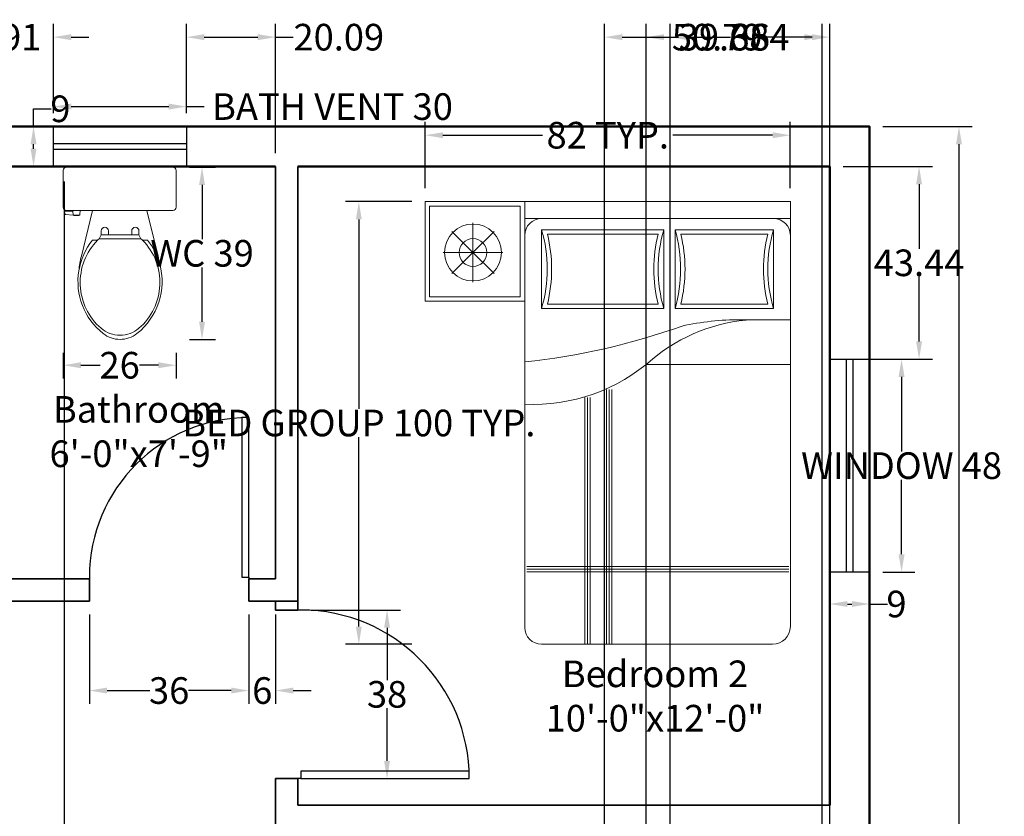
# Model space of a CAD drawing. Units: inches. Extents: x 89 to 490, y -59 to 378.
# Tile 20 of 20: x 268 to 490, y 198 to 378. Entities that reach past the tile are written whole.
import ezdxf

# ---------------------------------------------------------------- set-up
doc = ezdxf.new("R2010")
doc.units = ezdxf.units.IN
doc.header["$MEASUREMENT"] = 0
for name, color, linetype, lineweight in [('A-ANNO-DIMS', 2, 'Continuous', 18), ('A-AREA-IDEN', 7, 'Continuous', 18), ('Beds', 64, 'Continuous', 18), ('Commode', 232, 'Continuous', 18), ('Doors', 34, 'Continuous', 25), ('Inner Walls', 31, 'Continuous', 35), ('Outer Walls', 12, 'Continuous', 50), ('Ventilators', 130, 'Continuous', 25), ('Windows', 171, 'Continuous', 25)]:
    doc.layers.add(name, color=color, linetype=linetype, lineweight=lineweight)
doc.styles.get("Standard").update_dxf_attribs({"font": 'arial.ttf'})
doc.dimstyles.get("Standard").update_dxf_attribs({"dimtxt": 6, "dimasz": 4, "dimexe": 3, "dimexo": 3, "dimgap": 0.09, "dimtad": 0, "dimtih": 1, "dimtoh": 1, "dimdec": 1, "dimzin": 0, "dimdsep": 46, "dimlunit": 3, "dimtxsty": 'Standard', "dimcen": 0.09, "dimadec": 0, "dimazin": 0, "dimtfac": 1, "dimtdec": 1, "dimtofl": 0, "dimtmove": 0, "dimatfit": 3, "dimfxl": 1, "dimtolj": 1, "dimtzin": 0, "dimarcsym": 0})

# ---------------------------------------------------------------- blocks, each defined once
blk = doc.blocks.new('Ventilator')
for p, q in [((814.98, 322.93), (844.98, 322.93)), ((814.98, 313.93), (814.98, 322.93)), ((844.98, 322.93), (844.98, 313.93)), ((814.98, 319.13), (844.98, 319.13)), ((844.98, 317.73), (814.98, 317.73)), ((844.98, 313.93), (814.98, 313.93))]:
    blk.add_line(p, q)
blk = doc.blocks.new('Window 1.1')
for p, q in [((642.96, 338.61), (642.96, 386.61)), ((644.36, 386.61), (644.36, 338.61))]:
    blk.add_line(p, q)
blk.add_lwpolyline([(648.16, 338.61), (639.16, 338.61), (639.16, 386.61), (648.16, 386.61)], close=True)
blk = doc.blocks.new('*U8')
for p, q in [((0, 0), (0, 6)), ((40, 0), (40, 6))]:
    blk.add_line(p, q)
blk.add_lwpolyline([(0, 0), (0, -40), (1.75, -40), (1.75, 0)], close=True)
blk.add_arc((0, 0), 40, 270, 0)
blk = doc.blocks.new('*U7')
for p, q in [((0, 0), (0, -6)), ((-40, 0), (-40, -6))]:
    blk.add_line(p, q)
blk.add_lwpolyline([(0, 0), (0, 40), (-1.75, 40), (-1.75, 0)], close=True)
blk.add_arc((0, 0), 40, 90, 180)
blk = doc.blocks.new('A$C216962CD')
at = {"linetype": 'ByBlock'}
for p, q in [((0, 1.5502), (0, 2.0002)), ((0, 2.0002), (0.45, 2.0002)), ((0.45, 1.924), (0.45, 2.0002)), ((0.45, 2.0002), (0.45, 1.5502)), ((0.45, 2.0002), (1.6506, 2.0002)), ((1.6506, 2.0002), (1.6506, 1.5502)), ((0.45, 1.924), (1.6506, 1.924)), ((0.5262, 1.8732), (0.5262, 1.5176)), ((1.0785, 1.8732), (0.5262, 1.8732)), ((1.0785, 1.5176), (1.0785, 1.8732)), ((1.1293, 1.8732), (1.1293, 1.5176)), ((1.5744, 1.8732), (1.1293, 1.8732)), ((1.5744, 1.5176), (1.5744, 1.8732)), ((0.45, 0.0762), (0.45, 1.8478)), ((1.6506, 1.8478), (1.6506, 0.08)), ((0.45, 1.5502), (0, 1.5502)), ((0.5262, 1.5176), (1.0785, 1.5176)), ((1.1293, 1.5176), (1.5744, 1.5176)), ((1.4247, 1.4668), (1.6506, 1.4668)), ((1.0023, 1.2636), (1.6506, 1.2636)), ((1.5706, 0), (0.5262, 0))]:
    blk.add_line(p, q, dxfattribs=at)
for p, q in [((0.02, 1.5702), (0.02, 1.9802)), ((0.02, 1.9802), (0.43, 1.9802)), ((0.43, 1.9802), (0.43, 1.5702)), ((0.216, 1.7702), (0.216, 1.9046)), ((0.216, 1.7702), (0.121, 1.8652)), ((0.216, 1.7702), (0.3111, 1.8652)), ((1.0524, 1.8532), (0.5523, 1.8532)), ((1.5483, 1.8532), (1.1554, 1.8532)), ((0.216, 1.7702), (0.0817, 1.7702)), ((0.216, 1.7702), (0.121, 1.6752)), ((0.216, 1.7702), (0.216, 1.6358)), ((0.216, 1.7702), (0.3504, 1.7702)), ((0.216, 1.7702), (0.3111, 1.6752)), ((0.43, 1.5702), (0.02, 1.5702)), ((0.5523, 1.5376), (1.0524, 1.5376)), ((1.1554, 1.5376), (1.5483, 1.5376)), ((0.722, 1.1146), (0.722, 0)), ((0.734, 1.1146), (0.734, 0)), ((0.746, 1.1146), (0.746, 0)), ((0.8202, 1.1507), (0.8202, 0)), ((0.8322, 1.1507), (0.8322, 0)), ((0.8442, 1.1507), (0.8442, 0)), ((0.4599, 0.3521), (1.6437, 0.3521)), ((0.4599, 0.3401), (1.6437, 0.3401)), ((0.4599, 0.3281), (1.6437, 0.3281))]:
    blk.add_line(p, q)
for radius in [0.1285, 0.0628]:
    blk.add_circle((0.216, 1.7702), radius)
for centre, radius, start, end in [((0.5262, 1.8478), 0.0762, 90, 180), ((1.5744, 1.8478), 0.0762, 0, 90), ((-0.0834, 1.6954), 0.635, 343.7398, 16.2602), ((1.6881, 1.6954), 0.635, 163.7398, 196.2602), ((0.5197, 1.6954), 0.635, 343.7398, 16.2602), ((2.184, 1.6954), 0.635, 163.7398, 196.2602), ((0.1309, 4.3115), 3.0525, 275.9977, 289.7225), ((1.5209, 0.6982), 0.7696, 92.9261, 129.8555), ((1.4243, 0.2475), 1.2193, 89.9814, 102.4667), ((0.4856, 1.9017), 0.8181, 267.5082, 311.5038), ((0.5262, 0.0762), 0.0762, 180, 270), ((1.5706, 0.08), 0.08, 270, 0)]:
    blk.add_arc(centre, radius, start, end, dxfattribs=at)
for centre, start, end in [((-0.0834, 1.6954), 346.0594, 13.9406), ((1.6881, 1.6954), 166.0594, 193.9406), ((0.5197, 1.6954), 346.0594, 13.9406), ((2.184, 1.6954), 166.0594, 193.9406)]:
    blk.add_arc(centre, 0.655, start, end)
blk = doc.blocks.new('B1')
at = {"color": 0}
for p, q in [((0, 0), (-240, 0)), ((240, 0), (0, 0)), ((-255, -15), (-255, -180)), ((255, -180), (255, -15)), ((-212, -198.4), (-250.1, -198.4)), ((-250.1, -198.4), (-245.5, -212.1)), ((-243.7, -213.5), (-210.1, -215.4)), ((-240, -195), (-212.3, -195)), ((-212.3, -195), (-177.6, -195)), ((-212.3, -195), (-212, -198.4)), ((-212, -198.4), (-210.1, -215.4)), ((-206.1, -215.4), (-210.1, -215.4)), ((-206.1, -215.4), (-205.1, -217.4)), ((-184.1, -215.4), (-206.1, -215.4)), ((-185.1, -217.4), (-205.1, -217.4)), ((-184.1, -215.4), (-185.1, -217.4)), ((-181.8, -215.4), (-184.1, -215.4)), ((-177.6, -195), (-179.8, -213.7)), ((-177.6, -195), (-122, -195)), ((-122, -195), (-172.9, -400.4)), ((0, -195), (-122, -195)), ((122, -195), (0, -195)), ((172.9, -400.4), (122, -195)), ((122, -195), (240, -195)), ((-92.8, -322.2), (-83.7, -305.5)), ((-83.7, -305.5), (-83.7, -287.2)), ((-50.9, -305.5), (-83.7, -305.5)), ((-50.9, -287.2), (-50.9, -305.5)), ((1.6, -305.5), (-50.9, -305.5)), ((1.6, -305.5), (54.2, -305.5)), ((54.2, -287.2), (54.2, -305.5)), ((54.2, -305.5), (86.9, -305.5)), ((86.9, -305.5), (86.9, -287.2)), ((96.1, -322.2), (86.9, -305.5)), ((-99.8, -329.1), (-122.6, -329.1)), ((1.6, -322.2), (-92.8, -322.2)), ((1.6, -322.2), (96.1, -322.2)), ((103.1, -329.1), (125.8, -329.1))]:
    blk.add_line(p, q, dxfattribs=at)
for centre, radius, start, end in [((-240, -15), 15, 90, 180), ((240, -15), 15, 360, 90), ((-240, -180), 15, 180, 270), ((-243.6, -211.5), 2, 198.4349, 266.7295), ((-181.8, -213.4), 2, 270, 353.0073), ((240, -180), 15, 270, 0), ((-67.3, -287.2), 16.4, 0, 180), ((70.6, -287.2), 16.4, 0, 180), ((110.1, -515.7), 298.3, 141.274, 170.4901), ((93.8, -520.1), 272, 135.3828, 229.2681), ((93.8, -520.1), 272, 133.3236, 135.3828), ((-90.5, -520.1), 272, 310.7319, 44.6172), ((-90.5, -520.1), 272, 44.6172, 46.6764), ((-106.9, -515.7), 298.3, 15.5851, 38.726), ((175, -492.8), 360, 165.1314, 175.7954), ((-106.9, -515.7), 298.3, 308.2583, 15.5851), ((-175, -492.8), 360, 9.1506, 14.8686), ((110.1, -515.7), 298.3, 170.4901, 231.7417), ((0.1, -628.9), 128.5, 229.2681, 270.6684), ((1.7, -653.2), 123.1, 231.7417, 269.9885), ((3.1, -628.9), 128.5, 269.3316, 310.7319), ((1.6, -653.2), 123.1, 270.0115, 308.2583)]:
    blk.add_arc(centre, radius, start, end, dxfattribs=at)
blk = doc.blocks.new('*D24')
at = {"layer": 'A-ANNO-DIMS', "color": 0, "lineweight": -2, "transparency": 16777216}
for p, q in [((306.03, 344.57), (311.86, 344.57)), ((308.86, 340.57), (308.86, 328.35)), ((308.86, 309.75), (308.86, 321.96)), ((306.03, 305.75), (311.86, 305.75))]:
    blk.add_line(p, q, dxfattribs=at)
at = {"layer": 'A-ANNO-DIMS', "color": 0, "transparency": 16777216}
for points in [[(308.19, 340.57), (309.52, 340.57), (308.86, 344.57)], [(308.19, 309.75), (309.52, 309.75), (308.86, 305.75)]]:
    blk.add_solid(points, dxfattribs=at)
at = {"layer": 'Defpoints', "color": 0, "transparency": 16777216}
for p in [(303.03, 344.57), (308.86, 344.57), (303.03, 305.75)]:
    blk.add_point(p, dxfattribs=at)
at = {"layer": 'A-ANNO-DIMS', "color": 0, "transparency": 16777216, "insert": (308.86, 325.16), "char_height": 6, "attachment_point": 5}
blk.add_mtext('\\A1;WC 39', dxfattribs=at)
blk = doc.blocks.new('*D25')
at = {"layer": 'A-ANNO-DIMS', "color": 0, "lineweight": -2, "transparency": 16777216}
for p, q in [((277.53, 302.75), (277.53, 296.93)), ((303.03, 302.75), (303.03, 296.93)), ((281.53, 299.93), (285.85, 299.93)), ((299.03, 299.93), (294.72, 299.93))]:
    blk.add_line(p, q, dxfattribs=at)
at = {"layer": 'A-ANNO-DIMS', "color": 0, "transparency": 16777216}
for points in [[(281.53, 300.6), (281.53, 299.26), (277.53, 299.93)], [(299.03, 300.6), (299.03, 299.26), (303.03, 299.93)]]:
    blk.add_solid(points, dxfattribs=at)
at = {"layer": 'Defpoints', "color": 0, "transparency": 16777216}
for p in [(277.53, 305.75), (303.03, 305.75), (303.03, 299.93)]:
    blk.add_point(p, dxfattribs=at)
at = {"layer": 'A-ANNO-DIMS', "color": 0, "transparency": 16777216, "insert": (290.28, 299.93), "char_height": 6, "attachment_point": 5}
blk.add_mtext('\\A1;26', dxfattribs=at)
blk = doc.blocks.new('*D26')
at = {"layer": 'A-ANNO-DIMS', "color": 0, "lineweight": -2, "transparency": 16777216}
for p, q in [((275.35, 356.74), (275.35, 361.24)), ((305.35, 356.74), (305.35, 361.24)), ((279.35, 358.24), (301.35, 358.24)), ((305.35, 358.24), (309.35, 358.24))]:
    blk.add_line(p, q, dxfattribs=at)
at = {"layer": 'A-ANNO-DIMS', "color": 0, "transparency": 16777216}
for points in [[(279.35, 358.91), (279.35, 357.57), (275.35, 358.24)], [(301.35, 358.91), (301.35, 357.57), (305.35, 358.24)]]:
    blk.add_solid(points, dxfattribs=at)
at = {"layer": 'Defpoints', "color": 0, "transparency": 16777216}
for p in [(305.35, 358.24), (275.35, 353.74), (305.35, 353.74)]:
    blk.add_point(p, dxfattribs=at)
at = {"layer": 'A-ANNO-DIMS', "color": 0, "transparency": 16777216, "insert": (338.28, 358.24), "char_height": 6, "attachment_point": 5}
blk.add_mtext('\\A1;BATH VENT 30', dxfattribs=at)
blk = doc.blocks.new('*D27')
at = {"layer": 'A-ANNO-DIMS', "color": 0, "lineweight": -2, "transparency": 16777216}
for p, q in [((270.85, 353.74), (270.85, 357.74)), ((270.85, 357.74), (274.85, 357.74)), ((272.35, 353.74), (267.85, 353.74)), ((270.85, 348.74), (270.85, 349.74)), ((272.35, 344.74), (267.85, 344.74))]:
    blk.add_line(p, q, dxfattribs=at)
at = {"layer": 'A-ANNO-DIMS', "color": 0, "transparency": 16777216}
for points in [[(270.18, 349.74), (271.52, 349.74), (270.85, 353.74)], [(270.18, 348.74), (271.52, 348.74), (270.85, 344.74)]]:
    blk.add_solid(points, dxfattribs=at)
at = {"layer": 'Defpoints', "color": 0, "transparency": 16777216}
for p in [(270.85, 353.74), (275.35, 353.74), (275.35, 344.74)]:
    blk.add_point(p, dxfattribs=at)
at = {"layer": 'A-ANNO-DIMS', "color": 0, "transparency": 16777216, "insert": (276.91, 357.74), "char_height": 6, "attachment_point": 5}
blk.add_mtext('\\A1;9', dxfattribs=at)
blk = doc.blocks.new('*D30')
at = {"layer": 'A-ANNO-DIMS', "color": 0, "lineweight": -2, "transparency": 16777216}
for p, q in [((356.2, 336.82), (341.22, 336.82)), ((344.22, 332.82), (344.22, 290.11)), ((344.22, 241.01), (344.22, 283.72)), ((356.2, 237.01), (341.22, 237.01))]:
    blk.add_line(p, q, dxfattribs=at)
at = {"layer": 'A-ANNO-DIMS', "color": 0, "transparency": 16777216}
for points in [[(343.56, 332.82), (344.89, 332.82), (344.22, 336.82)], [(343.56, 241.01), (344.89, 241.01), (344.22, 237.01)]]:
    blk.add_solid(points, dxfattribs=at)
at = {"layer": 'Defpoints', "color": 0, "transparency": 16777216}
for p in [(344.22, 336.82), (359.2, 336.82), (359.2, 237.01)]:
    blk.add_point(p, dxfattribs=at)
at = {"layer": 'A-ANNO-DIMS', "color": 0, "transparency": 16777216, "insert": (344.22, 286.91), "char_height": 6, "attachment_point": 5}
blk.add_mtext('\\A1;BED GROUP 100 TYP.', dxfattribs=at)
blk = doc.blocks.new('*D31')
at = {"layer": 'A-ANNO-DIMS', "color": 0, "lineweight": -2, "transparency": 16777216}
for p, q in [((359.2, 339.82), (359.2, 354.79)), ((441.55, 339.82), (441.55, 354.79)), ((363.2, 351.79), (385.68, 351.79)), ((437.55, 351.79), (415.07, 351.79))]:
    blk.add_line(p, q, dxfattribs=at)
at = {"layer": 'A-ANNO-DIMS', "color": 0, "transparency": 16777216}
for points in [[(363.2, 352.45), (363.2, 351.12), (359.2, 351.79)], [(437.55, 352.45), (437.55, 351.12), (441.55, 351.79)]]:
    blk.add_solid(points, dxfattribs=at)
at = {"layer": 'Defpoints', "color": 0, "transparency": 16777216}
for p in [(441.55, 351.79), (359.2, 336.82), (441.55, 336.82)]:
    blk.add_point(p, dxfattribs=at)
at = {"layer": 'A-ANNO-DIMS', "color": 0, "transparency": 16777216, "insert": (400.37, 351.79), "char_height": 6, "attachment_point": 5}
blk.add_mtext('\\A1;82 TYP.', dxfattribs=at)
blk = doc.blocks.new('*D34')
at = {"layer": 'A-ANNO-DIMS', "color": 0, "lineweight": -2, "transparency": 16777216}
for p, q in [((462.44, 301.3), (469.64, 301.3)), ((466.64, 297.3), (466.64, 280.49)), ((466.64, 257.3), (466.64, 274.11)), ((462.44, 253.3), (469.64, 253.3))]:
    blk.add_line(p, q, dxfattribs=at)
at = {"layer": 'A-ANNO-DIMS', "color": 0, "transparency": 16777216}
for points in [[(465.97, 297.3), (467.31, 297.3), (466.64, 301.3)], [(465.97, 257.3), (467.31, 257.3), (466.64, 253.3)]]:
    blk.add_solid(points, dxfattribs=at)
at = {"layer": 'Defpoints', "color": 0, "transparency": 16777216}
for p in [(459.44, 301.3), (466.64, 301.3), (459.44, 253.3)]:
    blk.add_point(p, dxfattribs=at)
at = {"layer": 'A-ANNO-DIMS', "color": 0, "transparency": 16777216, "insert": (466.64, 277.3), "char_height": 6, "attachment_point": 5}
blk.add_mtext('\\A1;WINDOW 48', dxfattribs=at)
blk = doc.blocks.new('*D35')
at = {"layer": 'A-ANNO-DIMS', "color": 0, "lineweight": -2, "transparency": 16777216}
for p, q in [((450.44, 250.3), (450.44, 243.1)), ((459.44, 250.3), (459.44, 243.1)), ((454.44, 246.1), (455.44, 246.1)), ((459.44, 246.1), (463.44, 246.1))]:
    blk.add_line(p, q, dxfattribs=at)
at = {"layer": 'A-ANNO-DIMS', "color": 0, "transparency": 16777216}
for points in [[(454.44, 246.77), (454.44, 245.43), (450.44, 246.1)], [(455.44, 246.77), (455.44, 245.43), (459.44, 246.1)]]:
    blk.add_solid(points, dxfattribs=at)
at = {"layer": 'Defpoints', "color": 0, "transparency": 16777216}
for p in [(450.44, 253.3), (459.44, 253.3), (459.44, 246.1)]:
    blk.add_point(p, dxfattribs=at)
at = {"layer": 'A-ANNO-DIMS', "color": 0, "transparency": 16777216, "insert": (465.5, 246.1), "char_height": 6, "attachment_point": 5}
blk.add_mtext('\\A1;9', dxfattribs=at)
blk = doc.blocks.new('*D49')
at = {"layer": 'A-ANNO-DIMS', "color": 0, "lineweight": -2, "transparency": 16777216}
for p, q in [((462.44, 353.74), (482.59, 353.74)), ((479.59, 349.74), (479.59, 166.7)), ((479.59, -22.66), (479.59, 160.39)), ((462.44, -26.66), (482.59, -26.66))]:
    blk.add_line(p, q, dxfattribs=at)
at = {"layer": 'A-ANNO-DIMS', "color": 0, "transparency": 16777216}
for points in [[(478.92, 349.74), (480.26, 349.74), (479.59, 353.74)], [(478.92, -22.66), (480.26, -22.66), (479.59, -26.66)]]:
    blk.add_solid(points, dxfattribs=at)
at = {"layer": 'Defpoints', "color": 0, "transparency": 16777216}
for p in [(459.44, 353.74), (479.59, 353.74), (459.44, -26.66)]:
    blk.add_point(p, dxfattribs=at)
at = {"layer": 'A-ANNO-DIMS', "color": 0, "transparency": 16777216, "insert": (479.59, 163.54), "char_height": 6, "attachment_point": 5}
blk.add_mtext('\\A1;380.4', dxfattribs=at)
blk = doc.blocks.new('*D53')
at = {"layer": 'A-ANNO-DIMS', "color": 0, "lineweight": -2, "transparency": 16777216}
for p, q in [((249.44, 347.74), (249.44, 376.89)), ((275.35, 356.74), (275.35, 376.89)), ((245.44, 373.89), (241.44, 373.89)), ((279.35, 373.89), (283.35, 373.89))]:
    blk.add_line(p, q, dxfattribs=at)
at = {"layer": 'A-ANNO-DIMS', "color": 0, "transparency": 16777216}
for points in [[(245.44, 374.56), (245.44, 373.22), (249.44, 373.89)], [(279.35, 374.56), (279.35, 373.22), (275.35, 373.89)]]:
    blk.add_solid(points, dxfattribs=at)
at = {"layer": 'Defpoints', "color": 0, "transparency": 16777216}
for p in [(275.35, 373.89), (275.35, 353.74), (249.44, 344.74)]:
    blk.add_point(p, dxfattribs=at)
at = {"layer": 'A-ANNO-DIMS', "color": 0, "transparency": 16777216, "insert": (262.4, 373.89), "char_height": 6, "attachment_point": 5}
blk.add_mtext('\\A1;25.91', dxfattribs=at)
blk = doc.blocks.new('*D55')
at = {"layer": 'A-ANNO-DIMS', "color": 0, "lineweight": -2, "transparency": 16777216}
for p, q in [((305.35, 356.74), (305.35, 376.89)), ((325.44, 347.74), (325.44, 376.89)), ((309.35, 373.89), (321.44, 373.89)), ((325.44, 373.89), (329.44, 373.89))]:
    blk.add_line(p, q, dxfattribs=at)
at = {"layer": 'A-ANNO-DIMS', "color": 0, "transparency": 16777216}
for points in [[(309.35, 374.56), (309.35, 373.22), (305.35, 373.89)], [(321.44, 374.56), (321.44, 373.22), (325.44, 373.89)]]:
    blk.add_solid(points, dxfattribs=at)
at = {"layer": 'Defpoints', "color": 0, "transparency": 16777216}
for p in [(325.44, 373.89), (305.35, 353.74), (325.44, 344.74)]:
    blk.add_point(p, dxfattribs=at)
at = {"layer": 'A-ANNO-DIMS', "color": 0, "transparency": 16777216, "insert": (339.71, 373.89), "char_height": 6, "attachment_point": 5}
blk.add_mtext('\\A1;20.09', dxfattribs=at)
blk = doc.blocks.new('*D56')
at = {"layer": 'A-ANNO-DIMS', "color": 0, "lineweight": -2, "transparency": 16777216}
for p, q in [((414.44, 63.07), (414.44, 376.89)), ((450.44, 63.07), (450.44, 376.89)), ((418.44, 373.89), (428.06, 373.89)), ((446.44, 373.89), (436.82, 373.89))]:
    blk.add_line(p, q, dxfattribs=at)
at = {"layer": 'A-ANNO-DIMS', "color": 0, "transparency": 16777216}
for points in [[(418.44, 374.56), (418.44, 373.22), (414.44, 373.89)], [(446.44, 374.56), (446.44, 373.22), (450.44, 373.89)]]:
    blk.add_solid(points, dxfattribs=at)
at = {"layer": 'Defpoints', "color": 0, "transparency": 16777216}
for p in [(450.44, 373.89), (414.44, 60.07), (450.44, 60.07)]:
    blk.add_point(p, dxfattribs=at)
at = {"layer": 'A-ANNO-DIMS', "color": 0, "transparency": 16777216, "insert": (432.44, 373.89), "char_height": 6, "attachment_point": 5}
blk.add_mtext('\\A1;36', dxfattribs=at)
blk = doc.blocks.new('*D61')
at = {"layer": 'A-ANNO-DIMS', "color": 0, "lineweight": -2, "transparency": 16777216}
for p, q in [((333.44, 244.74), (353.59, 244.74)), ((350.59, 240.74), (350.59, 228.9)), ((350.59, 210.74), (350.59, 222.59)), ((333.44, 206.74), (353.59, 206.74))]:
    blk.add_line(p, q, dxfattribs=at)
at = {"layer": 'A-ANNO-DIMS', "color": 0, "transparency": 16777216}
for points in [[(349.92, 240.74), (351.26, 240.74), (350.59, 244.74)], [(349.92, 210.74), (351.26, 210.74), (350.59, 206.74)]]:
    blk.add_solid(points, dxfattribs=at)
at = {"layer": 'Defpoints', "color": 0, "transparency": 16777216}
for p in [(330.44, 244.74), (330.44, 206.74), (350.59, 206.74)]:
    blk.add_point(p, dxfattribs=at)
at = {"layer": 'A-ANNO-DIMS', "color": 0, "transparency": 16777216, "insert": (350.59, 225.74), "char_height": 6, "attachment_point": 5}
blk.add_mtext('\\A1;38', dxfattribs=at)
blk = doc.blocks.new('*D62')
at = {"layer": 'A-ANNO-DIMS', "color": 0, "lineweight": -2, "transparency": 16777216}
for p, q in [((283.44, 243.74), (283.44, 223.59)), ((319.44, 243.74), (319.44, 223.59)), ((287.44, 226.59), (297.06, 226.59)), ((315.44, 226.59), (305.82, 226.59))]:
    blk.add_line(p, q, dxfattribs=at)
at = {"layer": 'A-ANNO-DIMS', "color": 0, "transparency": 16777216}
for points in [[(287.44, 227.26), (287.44, 225.92), (283.44, 226.59)], [(315.44, 227.26), (315.44, 225.92), (319.44, 226.59)]]:
    blk.add_solid(points, dxfattribs=at)
at = {"layer": 'Defpoints', "color": 0, "transparency": 16777216}
for p in [(283.44, 246.74), (319.44, 246.74), (283.44, 226.59)]:
    blk.add_point(p, dxfattribs=at)
at = {"layer": 'A-ANNO-DIMS', "color": 0, "transparency": 16777216, "insert": (301.44, 226.59), "char_height": 6, "attachment_point": 5}
blk.add_mtext('\\A1;36', dxfattribs=at)
blk = doc.blocks.new('*D63')
at = {"layer": 'A-ANNO-DIMS', "color": 0, "lineweight": -2, "transparency": 16777216}
for p, q in [((319.44, 243.74), (319.44, 223.59)), ((325.44, 243.74), (325.44, 223.59)), ((315.44, 226.59), (311.44, 226.59)), ((329.44, 226.59), (333.44, 226.59))]:
    blk.add_line(p, q, dxfattribs=at)
at = {"layer": 'A-ANNO-DIMS', "color": 0, "transparency": 16777216}
for points in [[(315.44, 227.26), (315.44, 225.92), (319.44, 226.59)], [(329.44, 227.26), (329.44, 225.92), (325.44, 226.59)]]:
    blk.add_solid(points, dxfattribs=at)
at = {"layer": 'Defpoints', "color": 0, "transparency": 16777216}
for p in [(319.44, 246.74), (325.44, 246.74), (319.44, 226.59)]:
    blk.add_point(p, dxfattribs=at)
at = {"layer": 'A-ANNO-DIMS', "color": 0, "transparency": 16777216, "insert": (322.44, 226.59), "char_height": 6, "attachment_point": 5}
blk.add_mtext('\\A1;6', dxfattribs=at)
blk = doc.blocks.new('*D64')
at = {"layer": 'A-ANNO-DIMS', "color": 0, "lineweight": -2, "transparency": 16777216}
for p, q in [((399.65, 16.74), (399.65, 376.89)), ((450.44, 16.74), (450.44, 376.89)), ((403.65, 373.89), (414.83, 373.89)), ((446.44, 373.89), (435.27, 373.89))]:
    blk.add_line(p, q, dxfattribs=at)
at = {"layer": 'A-ANNO-DIMS', "color": 0, "transparency": 16777216}
for points in [[(403.65, 374.56), (403.65, 373.22), (399.65, 373.89)], [(446.44, 374.56), (446.44, 373.22), (450.44, 373.89)]]:
    blk.add_solid(points, dxfattribs=at)
at = {"layer": 'Defpoints', "color": 0, "transparency": 16777216}
for p in [(450.44, 373.89), (399.65, 13.74), (450.44, 13.74)]:
    blk.add_point(p, dxfattribs=at)
at = {"layer": 'A-ANNO-DIMS', "color": 0, "transparency": 16777216, "insert": (425.05, 373.89), "char_height": 6, "attachment_point": 5}
blk.add_mtext('\\A1;50.79', dxfattribs=at)
blk = doc.blocks.new('*D69')
at = {"layer": 'A-ANNO-DIMS', "color": 0, "lineweight": -2, "transparency": 16777216}
for p, q in [((453.44, 344.74), (473.59, 344.74)), ((470.59, 340.74), (470.59, 326.18)), ((470.59, 305.3), (470.59, 319.87)), ((453.44, 301.3), (473.59, 301.3))]:
    blk.add_line(p, q, dxfattribs=at)
at = {"layer": 'A-ANNO-DIMS', "color": 0, "transparency": 16777216}
for points in [[(469.92, 340.74), (471.26, 340.74), (470.59, 344.74)], [(469.92, 305.3), (471.26, 305.3), (470.59, 301.3)]]:
    blk.add_solid(points, dxfattribs=at)
at = {"layer": 'Defpoints', "color": 0, "transparency": 16777216}
for p in [(450.44, 344.74), (450.44, 301.3), (470.59, 301.3)]:
    blk.add_point(p, dxfattribs=at)
at = {"layer": 'A-ANNO-DIMS', "color": 0, "transparency": 16777216, "insert": (470.59, 323.02), "char_height": 6, "attachment_point": 5}
blk.add_mtext('\\A1;43.44', dxfattribs=at)
blk = doc.blocks.new('*D71')
at = {"layer": 'A-ANNO-DIMS', "color": 0, "lineweight": -2, "transparency": 16777216}
for p, q in [((409.04, 21.37), (409.04, 376.89)), ((448.72, 21.37), (448.72, 376.89)), ((413.04, 373.89), (416.35, 373.89)), ((444.72, 373.89), (441.41, 373.89))]:
    blk.add_line(p, q, dxfattribs=at)
at = {"layer": 'A-ANNO-DIMS', "color": 0, "transparency": 16777216}
for points in [[(413.04, 374.56), (413.04, 373.22), (409.04, 373.89)], [(444.72, 374.56), (444.72, 373.22), (448.72, 373.89)]]:
    blk.add_solid(points, dxfattribs=at)
at = {"layer": 'Defpoints', "color": 0, "transparency": 16777216}
for p in [(448.72, 373.89), (409.04, 18.37), (448.72, 18.37)]:
    blk.add_point(p, dxfattribs=at)
at = {"layer": 'A-ANNO-DIMS', "color": 0, "transparency": 16777216, "insert": (428.88, 373.89), "char_height": 6, "attachment_point": 5}
blk.add_mtext('\\A1;39.684', dxfattribs=at)
blk = doc.blocks.new('*D74')
at = {"layer": 'A-ANNO-DIMS', "color": 0, "lineweight": -2, "transparency": 16777216}
for p, q in [((249.44, 341.74), (249.44, -49.81)), ((277.75, 341.35), (277.75, -49.81)), ((253.44, -46.81), (253.91, -46.81)), ((273.75, -46.81), (273.28, -46.81))]:
    blk.add_line(p, q, dxfattribs=at)
at = {"layer": 'A-ANNO-DIMS', "color": 0, "transparency": 16777216}
for points in [[(253.44, -46.14), (253.44, -47.48), (249.44, -46.81)], [(273.75, -46.14), (273.75, -47.48), (277.75, -46.81)]]:
    blk.add_solid(points, dxfattribs=at)
at = {"layer": 'Defpoints', "color": 0, "transparency": 16777216}
for p in [(249.44, 344.74), (277.75, 344.35), (277.75, -46.81)]:
    blk.add_point(p, dxfattribs=at)
at = {"layer": 'A-ANNO-DIMS', "color": 0, "transparency": 16777216, "insert": (263.6, -46.81), "char_height": 6, "attachment_point": 5}
blk.add_mtext('\\A1;28.31', dxfattribs=at)

msp = doc.modelspace()

# ---------------------------------------------------------------- linework, layer by layer
at = {"layer": 'Inner Walls'}
for p, q in [((325.4414, 251.7413), (325.4414, 344.7413)), ((330.4414, 244.7413), (330.4414, 344.7413)), ((249.4414, 251.7413), (283.4414, 251.7413)), ((283.4414, 246.7413), (283.4414, 251.7413)), ((319.4414, 246.7413), (319.4414, 251.7413)), ((319.4414, 251.7413), (325.4414, 251.7413)), ((244.4414, 246.7413), (283.4414, 246.7413)), ((319.4414, 246.7413), (330.4414, 246.7413)), ((325.4414, 244.7413), (325.4414, 246.7413)), ((325.4414, 244.7413), (330.4414, 244.7413)), ((325.4414, 195.7413), (325.4414, 206.7413)), ((325.4414, 206.7413), (330.4414, 206.7413)), ((330.4414, 200.7413), (330.4414, 206.7413)), ((330.4414, 200.7413), (450.4414, 200.7413))]:
    msp.add_line(p, q, dxfattribs=at)
at = {"layer": 'Outer Walls'}
for p, q in [((249.4414, 344.7413), (325.4414, 344.7413)), ((330.4414, 344.7413), (450.4414, 344.7413)), ((450.4414, 200.7413), (450.4414, 344.7413))]:
    msp.add_line(p, q, dxfattribs=at)
msp.add_lwpolyline([(214.6478, 67.7413), (265.4414, 67.7413), (265.4414, 4.7413), (459.4414, 4.7413), (459.4414, 353.7413), (127.4414, 353.7413), (127.4414, 13.7413)], dxfattribs=at)

# ---------------------------------------------------------------- block references
at = {"layer": 'Beds', "xscale": 49.89604989604899, "yscale": 49.89604989604899, "zscale": 49.89604989604899}
msp.add_blockref('A$C216962CD', (359.1952, 237.014), dxfattribs=at)
at = {"layer": 'Commode', "xscale": 0.050000000000097, "yscale": 0.050000000000097, "zscale": 0.050000000000097}
msp.add_blockref('B1', (290.2838, 344.5665), dxfattribs=at)
at = {"layer": 'Doors', "xscale": 0.8999999999999989, "yscale": 0.8999999999999989, "zscale": 0.8999999999999989}
msp.add_blockref('*U7', (319.4414, 252.1413), dxfattribs=at)
at = {"layer": 'Doors', "xscale": 0.95, "yscale": 0.95, "zscale": 0.95, "rotation": 90}
msp.add_blockref('*U8', (331.1414, 206.7413), dxfattribs=at)
at = {"layer": 'Ventilators'}
msp.add_blockref('Ventilator', (-539.6343, 30.8145), dxfattribs=at)
at = {"layer": 'Windows'}
msp.add_blockref('Window 1.1', (-188.7147, -85.3119), dxfattribs=at)

# ---------------------------------------------------------------- texts
at = {"layer": 'A-AREA-IDEN', "char_height": 6, "attachment_point": 1}
for s, insert in [('\\pxqc;Bathroom\\P6\'-0"x7\'-9"', (271.372, 292.9751)), ('\\pxqc;Bedroom 2\\P10\'-0"x12\'-0"', (387.831, 233.3567))]:
    msp.add_mtext_dynamic_manual_height_columns(s, width=46.403971, gutter_width=1, heights=[0], dxfattribs=dict(at, insert=insert))

# ---------------------------------------------------------------- dimensions: what is measured, and where the dimension line sits
at = {"layer": 'A-ANNO-DIMS'}
for base, p1, p2, override, picture, middle in [((275.3499, 373.8913), (249.4414, 344.7413), (275.3499, 353.7413), {"dimdec": 2, "dimlfac": 1, "dimrnd": 0, "dimzin": 0, "dimdsep": 46, "dimlunit": 2}, '*D53', (262.3956, 373.8913)), ((325.4414, 373.8913), (305.3499, 353.7413), (325.4414, 344.7413), {"dimdec": 2, "dimlfac": 1, "dimrnd": 0, "dimzin": 0, "dimdsep": 46, "dimlunit": 2}, '*D55', (339.7122, 373.8913)), ((450.4414, 373.8913), (399.6539, 13.7413), (450.4414, 13.7413), {"dimdec": 2, "dimlfac": 1, "dimrnd": 0, "dimzin": 0, "dimdsep": 46, "dimlunit": 2}, '*D64', (425.0477, 373.8913)), ((448.7229, 373.8913), (409.0388, 18.3742), (448.7229, 18.3742), {"dimdec": 3, "dimlfac": 1, "dimrnd": 0, "dimzin": 0, "dimdsep": 46, "dimlunit": 2}, '*D71', (428.8809, 373.8913)), ((450.4414, 373.8913), (414.4414, 60.0723), (450.4414, 60.0723), {"dimdec": 0, "dimlfac": 1, "dimrnd": 0, "dimzin": 0, "dimdsep": 46, "dimlunit": 2}, '*D56', (432.4414, 373.8913)), ((277.7535, -46.8094), (249.4414, 344.7413), (277.7535, 344.3468), {"dimdec": 2, "dimlfac": 1, "dimrnd": 0, "dimzin": 0, "dimdsep": 46, "dimlunit": 2}, '*D74', (263.5974, -46.8094)), ((303.0338130014, 299.9290434613), (277.5338130013, 305.7513190676), (303.0338130014, 305.7513190676), {"dimdec": 0, "dimlfac": 1, "dimrnd": 0, "dimzin": 0, "dimdsep": 46, "dimlunit": 2}, '*D25', (290.2838130013, 299.9290434613)), ((459.4414, 246.1003), (450.4414, 253.3003), (459.4414, 253.3003), {"dimdec": 0, "dimlfac": 1, "dimrnd": 0, "dimzin": 0, "dimdsep": 46, "dimlunit": 2}, '*D35', (465.5041, 246.1003))]:
    dim = msp.add_linear_dim(base=base, p1=p1, p2=p2, dimstyle='Standard', override=override, dxfattribs=at)
    dim.commit()
    dim.dimension.update_dxf_attribs({"geometry": picture, "text_midpoint": middle})
for base, p1, p2, text, picture, middle in [((305.3499, 358.2413), (275.3499, 353.7413), (305.3499, 353.7413), 'BATH VENT <>', '*D26', (338.2775, 358.2413)), ((441.5536, 351.7864), (359.1952, 336.816), (441.5536, 336.816), '<> TYP.', '*D31', (400.3744, 351.7864))]:
    dim = msp.add_linear_dim(base=base, p1=p1, p2=p2, text=text, dimstyle='Standard', override={"dimdec": 0, "dimlfac": 1, "dimrnd": 0, "dimzin": 0, "dimdsep": 46, "dimlunit": 2}, dxfattribs=at)
    dim.commit()
    dim.dimension.update_dxf_attribs({"geometry": picture, "text_midpoint": middle})
for base, p1, p2, angle, override, picture, middle in [((270.8499, 353.7413), (275.3499, 344.7413), (275.3499, 353.7413), 90, {"dimdec": 0, "dimlfac": 1, "dimrnd": 0, "dimzin": 0, "dimdsep": 46, "dimlunit": 2}, '*D27', (276.9126, 357.7413)), ((479.5914, 353.7413), (459.4414, -26.6594), (459.4414, 353.7413), 90, {"dimdec": 1, "dimlfac": 1, "dimrnd": 0, "dimzin": 0, "dimdsep": 46, "dimlunit": 2}, '*D49', (479.5914, 163.5409)), ((470.5914, 301.3003), (450.4414, 344.7413), (450.4414, 301.3003), 270, {"dimdec": 2, "dimlfac": 1, "dimrnd": 0, "dimzin": 0, "dimdsep": 46, "dimlunit": 2}, '*D69', (470.5914, 323.0208)), ((283.4414, 226.5913), (319.4414, 246.7413), (283.4414, 246.7413), 180, {"dimdec": 0, "dimlfac": 1, "dimrnd": 0, "dimzin": 0, "dimdsep": 46, "dimlunit": 2}, '*D62', (301.4414, 226.5913)), ((319.4414, 226.5913), (325.4414, 246.7413), (319.4414, 246.7413), 180, {"dimdec": 0, "dimlfac": 1, "dimrnd": 0, "dimzin": 0, "dimdsep": 46, "dimlunit": 2}, '*D63', (322.4414, 226.5913)), ((350.5914, 206.7413), (330.4414, 244.7413), (330.4414, 206.7413), 270, {"dimdec": 0, "dimlfac": 1, "dimrnd": 0, "dimzin": 0, "dimdsep": 46, "dimlunit": 2}, '*D61', (350.5914, 225.7413))]:
    dim = msp.add_linear_dim(base=base, p1=p1, p2=p2, angle=angle, dimstyle='Standard', override=override, dxfattribs=at)
    dim.commit()
    dim.dimension.update_dxf_attribs({"geometry": picture, "text_midpoint": middle})
for base, p1, p2, text, picture, middle in [((308.8561, 344.5665), (303.0338, 305.7513), (303.0338, 344.5665), 'WC <>', '*D24', (308.8561, 325.1589)), ((344.2249, 336.816), (359.1952, 237.014), (359.1952, 336.816), 'BED GROUP <> TYP.', '*D30', (344.2249, 286.915)), ((466.6414, 301.3003), (459.4414, 253.3003), (459.4414, 301.3003), 'WINDOW <>', '*D34', (466.6414, 277.3003))]:
    dim = msp.add_linear_dim(base=base, p1=p1, p2=p2, angle=90, text=text, dimstyle='Standard', override={"dimdec": 0, "dimlfac": 1, "dimrnd": 0, "dimzin": 0, "dimdsep": 46, "dimlunit": 2}, dxfattribs=at)
    dim.commit()
    dim.dimension.update_dxf_attribs({"geometry": picture, "text_midpoint": middle})

doc.saveas('drawing.dxf')
